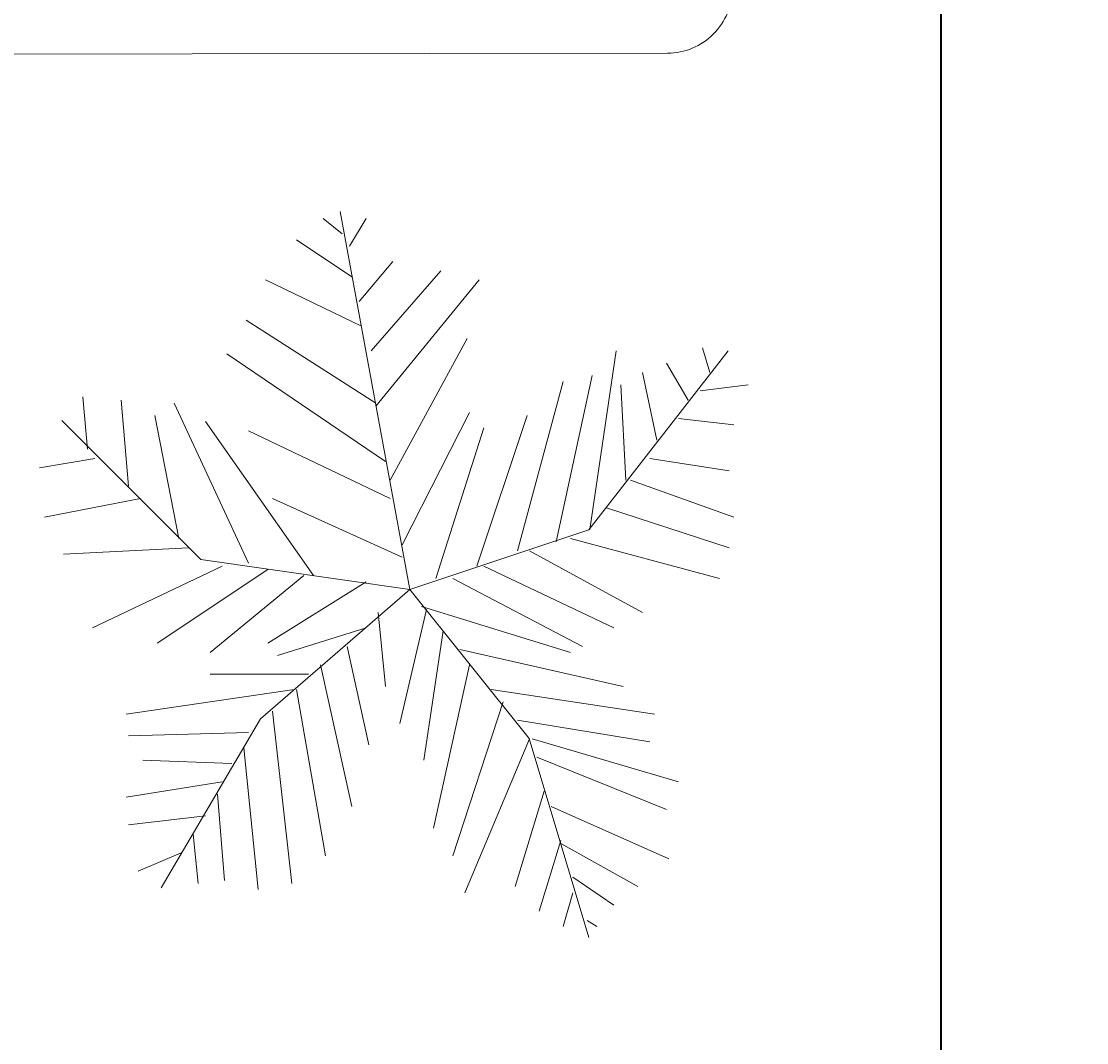
# Model space of a CAD drawing. Units: inches. Extents: x -61 to 1599, y -1316 to 257.
# Tile 135 of 204: x 507 to 540, y -166 to -135. Entities that reach past the tile are written whole.
import ezdxf

# ---------------------------------------------------------------- set-up
doc = ezdxf.new("R2010")
doc.units = ezdxf.units.IN
doc.header["$MEASUREMENT"] = 0
for name, color, linetype, lineweight in [('A-ANNO-DIMS', 2, 'Continuous', 18), ('FURNITURE', 83, 'Continuous', 18), ('WALLS', 4, 'Continuous', 35)]:
    doc.layers.add(name, color=color, linetype=linetype, lineweight=lineweight)
doc.styles.get("Standard").update_dxf_attribs({"font": 'arial.ttf'})
doc.dimstyles.get("Standard").update_dxf_attribs({"dimtxt": 0.18, "dimasz": 0.18, "dimexe": 0.18, "dimexo": 0.0625, "dimgap": 0.09, "dimtad": 0, "dimtih": 1, "dimtoh": 1, "dimdec": 0, "dimzin": 0, "dimdsep": 46, "dimlunit": 3, "dimtxsty": 'Standard', "dimcen": 0.09, "dimadec": 0, "dimazin": 0, "dimtfac": 1, "dimtdec": 0, "dimtofl": 0, "dimtmove": 0, "dimatfit": 3, "dimfxl": 1, "dimtolj": 1, "dimtzin": 0, "dimarcsym": 0})

# ---------------------------------------------------------------- blocks, each defined once
blk = doc.blocks.new('*U264')
for p, q in [((0, 0), (-10.5, 57)), ((-10.186, 53.64), (-13.084, 55.962)), ((-9.099, 51.782), (-6.563, 55.962)), ((-8.737, 47.138), (-17.069, 52.711)), ((-7.65, 43.423), (-2.578, 49.46)), ((-7.288, 39.707), (-21.778, 46.673)), ((-5.839, 35.992), (4.667, 48.067)), ((-5.114, 27.632), (10.463, 46.673)), ((-5.114, 28.097), (-24.676, 40.636)), ((-2.941, 16.486), (8.652, 37.85)), ((-3.665, 19.273), (-27.574, 35.527)), ((27, 9), (48, 36)), ((27.127, 9.056), (31.112, 35.992)), ((44.153, 36.456), (45.239, 32.741)), ((38.719, 34.134), (41.979, 28.561)), ((22.055, 7.198), (27.489, 32.277)), ((35.096, 32.741), (37.27, 22.524)), ((16.259, 5.805), (23.142, 31.348)), ((31.836, 30.883), (32.561, 16.486)), ((43.791, 29.954), (51.036, 30.883)), ((-48.585, 21.131), (-49.309, 29.026)), ((-43.513, 28.561), (-42.427, 15.558)), ((-35.544, 28.097), (-24.314, 3.947)), ((-38.442, 26.239), (-34.819, 7.663)), ((-1.129, 6.734), (9.014, 26.704)), ((10.101, 3.483), (17.708, 26.239)), ((40.53, 25.775), (48.862, 24.846)), ((-31.5, 4.5), (-52.5, 25.5)), ((-14.533, 2.09), (-30.834, 25.31)), ((3.942, 1.625), (11.187, 24.381)), ((-24.314, 23.917), (-2.941, 13.7)), ((-47.498, 19.737), (-55.83, 18.344)), ((36.183, 19.737), (48.137, 17.88)), ((33.285, 16.486), (48.862, 10.913)), ((-40.615, 13.7), (-55.105, 10.913)), ((-20.691, 13.7), (-1.129, 4.876)), ((29.662, 12.307), (48.137, 6.269)), ((0, 0), (27, 9)), ((24.229, 7.663), (46.688, 1.625)), ((-33.37, 6.269), (-52.207, 5.34)), ((18.07, 5.805), (35.096, -3.483)), ((-28.299, 3.483), (-47.86, -5.805)), ((0, 0), (-31.5, 4.5)), ((11.187, 3.483), (30.749, -5.805)), ((-21.416, 3.018), (-38.079, -8.128)), ((-15.982, 2.09), (-30.11, -9.521)), ((6.478, 1.625), (26.04, -8.592)), ((0, 0), (-22.5, -19.5)), ((-6.563, 1.161), (-21.416, -8.128)), ((0, 0), (18, -22.5)), ((2.493, -3.019), (-1.491, -20.202)), ((1.769, -2.555), (24.229, -9.521)), ((-4.752, -3.483), (-3.665, -14.629)), ((-6.563, -5.805), (-19.967, -9.985)), ((5.029, -6.27), (2.131, -25.775)), ((-9.461, -8.592), (-6.201, -23.453)), ((7.565, -9.056), (32.198, -14.629)), ((-15.257, -12.772), (-30.11, -12.772)), ((-13.446, -11.378), (-8.737, -32.741)), ((9.014, -11.378), (3.58, -35.992)), ((-17.431, -15.094), (-42.789, -18.809)), ((-17.069, -15.094), (-12.721, -40.172)), ((12.274, -15.094), (36.907, -18.809)), ((14.085, -16.951), (6.478, -40.172)), ((-20.691, -18.345), (-17.793, -44.352)), ((-22.5, -19.5), (-37.5, -45)), ((16.259, -19.738), (36.183, -22.989)), ((-24.314, -21.596), (-42.427, -22.06)), ((-25.038, -23.918), (-22.865, -45.281)), ((18.07, -22.524), (8.289, -45.745)), ((18, -22.5), (27, -52.5)), ((18.433, -22.524), (40.53, -29.026)), ((19.157, -25.311), (38.719, -33.206)), ((-26.849, -26.24), (-40.253, -25.775)), ((-28.299, -29.026), (-42.789, -31.348)), ((20.244, -30.419), (15.897, -44.816)), ((-29.023, -30.884), (-27.936, -43.887)), ((21.331, -32.741), (39.081, -40.636)), ((-30.834, -34.135), (-42.427, -35.528)), ((-32.646, -36.921), (-31.921, -44.352)), ((22.78, -37.85), (19.519, -48.532)), ((22.78, -38.314), (34.372, -44.816)), ((-34.457, -39.708), (-40.978, -42.494)), ((24.591, -43.423), (30.749, -47.603)), ((24.591, -45.745), (23.142, -50.854)), ((26.764, -49.925), (28.213, -50.854))]:
    blk.add_line(p, q)
blk = doc.blocks.new('*D704')
at = {"layer": 'A-ANNO-DIMS', "color": 0, "lineweight": -2, "transparency": 16777216}
for p, q in [((491.833, -616.882), (491.833, 257.457)), ((492.013, 257.277), (517.874, 257.277)), ((544.523, 257.277), (518.661, 257.277)), ((544.703, -616.882), (544.703, 257.457))]:
    blk.add_line(p, q, dxfattribs=at)
at = {"layer": 'A-ANNO-DIMS', "color": 0, "transparency": 16777216}
for points in [[(492.013, 257.307), (492.013, 257.247), (491.833, 257.277)], [(544.523, 257.307), (544.523, 257.247), (544.703, 257.277)]]:
    blk.add_solid(points, dxfattribs=at)
at = {"layer": 'DEFPOINTS', "color": 0, "transparency": 16777216}
for p in [(544.703, 257.277), (491.833, -616.945), (544.703, -616.945)]:
    blk.add_point(p, dxfattribs=at)
at = {"layer": 'A-ANNO-DIMS', "color": 0, "transparency": 16777216, "insert": (518.268, 257.277), "char_height": 0.18, "attachment_point": 5}
blk.add_mtext('\\A1;52.87', dxfattribs=at)

msp = doc.modelspace()

# ---------------------------------------------------------------- linework, layer by layer
at = {"layer": 'FURNITURE'}
msp.add_lwpolyline([(503.2659, -129.8197), (503.2714, -133.8197, 0.4142136), (505.2742, -135.817), (527.2741, -135.7867, 0.4142137), (529.2714, -133.784), (529.1944, -77.784, 0.4142134), (527.1916, -75.7868), (505.1917, -75.817, 0.4142136), (503.1944, -77.8197), (503.1999, -81.8197)], format="xyb", dxfattribs=at)
at = {"layer": 'WALLS'}
msp.add_line((535.7028, -13.3229), (535.7028, -175.3229), dxfattribs=at)

# ---------------------------------------------------------------- block references
at = {"layer": 'FURNITURE', "xscale": 0.2045054661246738, "yscale": 0.2045054661246738, "zscale": 0.2045054661246738}
msp.add_blockref('*U264', (519.3277, -152.3267), dxfattribs=at)

# ---------------------------------------------------------------- dimensions: what is measured, and where the dimension line sits
at = {"layer": 'A-ANNO-DIMS'}
dim = msp.add_linear_dim(base=(544.7028, 257.2771), p1=(491.8327, -616.9446), p2=(544.7028, -616.9446), dimstyle='Standard', override={"dimdec": 2, "dimlfac": 1, "dimrnd": 0, "dimzin": 0, "dimdsep": 46, "dimlunit": 2}, dxfattribs=at)
dim.commit()
dim.dimension.update_dxf_attribs({"geometry": '*D704', "text_midpoint": (518.2677, 257.2771)})

doc.saveas('drawing.dxf')
